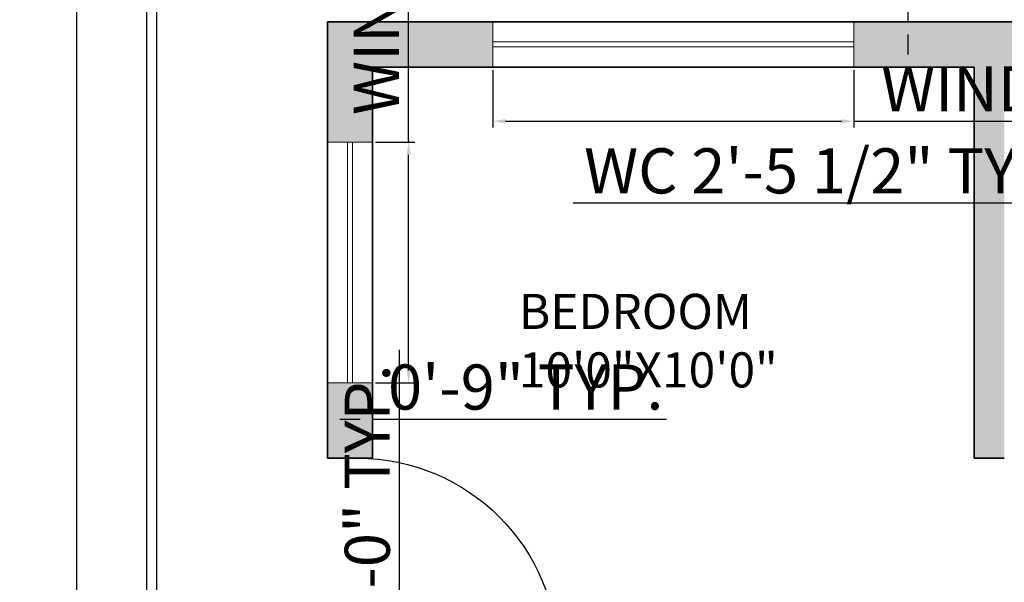
# Model space of a CAD drawing. Units: inches. Extents: x 2831 to 4250, y 1103 to 1797.
# Tile 3 of 15: x 3418 to 3614, y 1578 to 1690. Entities that reach past the tile are written whole.
import ezdxf

# ---------------------------------------------------------------- set-up
doc = ezdxf.new("R2010")
doc.units = ezdxf.units.IN
for name, color, linetype, lineweight in [('A-ANNO-DIMS', 2, 'Continuous', 18), ('A-AREA-IDEN', 7, 'Continuous', 18), ('A-DOOR', 4, 'Continuous', 25), ('A-WALL', 7, 'Continuous', 35), ('A-WALL-PATT', 252, 'Continuous', 13), ('C-PROP', 7, 'Continuous', 25), ('window', 130, 'Continuous', 18)]:
    doc.layers.add(name, color=color, linetype=linetype, lineweight=lineweight)
doc.styles.get("Standard").update_dxf_attribs({"font": 'arial.ttf'})
doc.dimstyles.new('ISO-25', dxfattribs={"dimtxt": 9, "dimasz": 2.5, "dimexe": 1.25, "dimexo": 0.625, "dimtad": 1, "dimdec": 1, "dimlunit": 3, "dimtxsty": 'Standard', "dimcen": 2.5, "dimadec": 0, "dimazin": 0, "dimtfac": 1, "dimtdec": 1, "dimtmove": 0, "dimatfit": 3, "dimfxl": 1, "dimarcsym": 0})

# ---------------------------------------------------------------- blocks, each defined once
blk = doc.blocks.new('*U2')
for p, q in [((0, 0), (0, -6)), ((40, 0), (40, -6))]:
    blk.add_line(p, q)
blk.add_lwpolyline([(0, 0), (0, 40), (1.75, 40), (1.75, 0)], close=True)
blk.add_arc((0, 0), 40, 0, 90)
blk = doc.blocks.new('*D6')
at = {"layer": 'A-ANNO-DIMS', "color": 0, "lineweight": -2, "transparency": 16777216}
for p, q in [((3442.6, 1722.51), (3427.96, 1722.51)), ((3429.21, 1720.01), (3429.21, 1245.01)), ((3442.6, 1242.51), (3427.96, 1242.51))]:
    blk.add_line(p, q, dxfattribs=at)
at = {"layer": 'A-ANNO-DIMS', "color": 0, "transparency": 16777216}
for points in [[(3428.79, 1720.01), (3429.62, 1720.01), (3429.21, 1722.51)], [(3428.79, 1245.01), (3429.62, 1245.01), (3429.21, 1242.51)]]:
    blk.add_solid(points, dxfattribs=at)
at = {"layer": 'Defpoints', "color": 0, "transparency": 16777216}
for p in [(3443.23, 1722.51), (3429.21, 1242.51), (3443.23, 1242.51)]:
    blk.add_point(p, dxfattribs=at)
at = {"layer": 'A-ANNO-DIMS', "color": 0, "transparency": 16777216, "insert": (3423.99, 1482.51), "char_height": 9, "attachment_point": 5, "rotation": 90}
blk.add_mtext("40'", dxfattribs=at)
blk = doc.blocks.new('WIN-48IN')
for p, q in [((9, 48), (0, 48)), ((4, 0), (4, 48)), ((5, 0), (5, 48)), ((9, 0), (0, 0))]:
    blk.add_line(p, q)
blk = doc.blocks.new('WIN-72IN')
for p, q in [((0, 0), (0, 9)), ((72, 0), (72, 9)), ((0, 5), (72, 5)), ((0, 4), (72, 4))]:
    blk.add_line(p, q)
blk = doc.blocks.new('*D73')
at = {"layer": 'A-ANNO-DIMS', "color": 0, "lineweight": -2, "transparency": 16777216}
for p, q in [((3495.43, 1665.51), (3495.43, 1783.15)), ((3488.85, 1665.51), (3496.68, 1665.51)), ((3495.43, 1620.01), (3495.43, 1663.01)), ((3488.85, 1617.51), (3496.68, 1617.51))]:
    blk.add_line(p, q, dxfattribs=at)
at = {"layer": 'A-ANNO-DIMS', "color": 0, "transparency": 16777216}
for points in [[(3495.01, 1663.01), (3495.84, 1663.01), (3495.43, 1665.51)], [(3495.01, 1620.01), (3495.84, 1620.01), (3495.43, 1617.51)]]:
    blk.add_solid(points, dxfattribs=at)
at = {"layer": 'Defpoints', "color": 0, "transparency": 16777216}
for p in [(3488.23, 1665.51), (3495.43, 1665.51), (3488.23, 1617.51)]:
    blk.add_point(p, dxfattribs=at)
at = {"layer": 'A-ANNO-DIMS', "color": 0, "transparency": 16777216, "insert": (3490.15, 1725.58), "char_height": 9, "attachment_point": 5, "rotation": 90}
blk.add_mtext('WINDOW 4\'-0" TYP.', dxfattribs=at)
blk = doc.blocks.new('*D74')
at = {"layer": 'A-ANNO-DIMS', "color": 0, "lineweight": -2, "transparency": 16777216}
for p, q in [((3479.23, 1616.89), (3479.23, 1609.06)), ((3488.23, 1616.89), (3488.23, 1609.06)), ((3481.73, 1610.31), (3485.73, 1610.31)), ((3488.23, 1610.31), (3546.84, 1610.31))]:
    blk.add_line(p, q, dxfattribs=at)
at = {"layer": 'A-ANNO-DIMS', "color": 0, "transparency": 16777216}
for points in [[(3481.73, 1610.73), (3481.73, 1609.9), (3479.23, 1610.31)], [(3485.73, 1610.73), (3485.73, 1609.9), (3488.23, 1610.31)]]:
    blk.add_solid(points, dxfattribs=at)
at = {"layer": 'Defpoints', "color": 0, "transparency": 16777216}
for p in [(3479.23, 1617.51), (3488.23, 1617.51), (3488.23, 1610.31)]:
    blk.add_point(p, dxfattribs=at)
at = {"layer": 'A-ANNO-DIMS', "color": 0, "transparency": 16777216, "insert": (3518.78, 1615.53), "char_height": 9, "attachment_point": 5}
blk.add_mtext('0\'-9" TYP.', dxfattribs=at)
blk = doc.blocks.new('*D75')
at = {"layer": 'A-ANNO-DIMS', "color": 0, "lineweight": -2, "transparency": 16777216}
for p, q in [((3493.63, 1506.51), (3493.63, 1624.15)), ((3488.85, 1506.51), (3494.88, 1506.51)), ((3493.63, 1473.01), (3493.63, 1504.01)), ((3488.85, 1470.51), (3494.88, 1470.51))]:
    blk.add_line(p, q, dxfattribs=at)
at = {"layer": 'A-ANNO-DIMS', "color": 0, "transparency": 16777216}
for points in [[(3493.21, 1504.01), (3494.04, 1504.01), (3493.63, 1506.51)], [(3493.21, 1473.01), (3494.04, 1473.01), (3493.63, 1470.51)]]:
    blk.add_solid(points, dxfattribs=at)
at = {"layer": 'Defpoints', "color": 0, "transparency": 16777216}
for p in [(3488.23, 1506.51), (3493.63, 1506.51), (3488.23, 1470.51)]:
    blk.add_point(p, dxfattribs=at)
at = {"layer": 'A-ANNO-DIMS', "color": 0, "transparency": 16777216, "insert": (3488.34, 1566.58), "char_height": 9, "attachment_point": 5, "rotation": 90}
blk.add_mtext('WINDOW 3\'-0" TYP.', dxfattribs=at)
blk = doc.blocks.new('*D77')
at = {"layer": 'A-ANNO-DIMS', "color": 0, "lineweight": -2, "transparency": 16777216}
for p, q in [((3512.23, 1679.89), (3512.23, 1668.46)), ((3584.23, 1679.89), (3584.23, 1668.46)), ((3514.73, 1669.71), (3581.73, 1669.71)), ((3584.23, 1669.71), (3701.86, 1669.71))]:
    blk.add_line(p, q, dxfattribs=at)
at = {"layer": 'A-ANNO-DIMS', "color": 0, "transparency": 16777216}
for points in [[(3514.73, 1670.13), (3514.73, 1669.3), (3512.23, 1669.71)], [(3581.73, 1670.13), (3581.73, 1669.3), (3584.23, 1669.71)]]:
    blk.add_solid(points, dxfattribs=at)
at = {"layer": 'Defpoints', "color": 0, "transparency": 16777216}
for p in [(3512.23, 1680.51), (3584.23, 1680.51), (3584.23, 1669.71)]:
    blk.add_point(p, dxfattribs=at)
at = {"layer": 'A-ANNO-DIMS', "color": 0, "transparency": 16777216, "insert": (3644.3, 1674.99), "char_height": 9, "attachment_point": 5}
blk.add_mtext('WINDOW 6\'-0" TYP.', dxfattribs=at)
blk = doc.blocks.new('*D78')
at = {"layer": 'A-ANNO-DIMS', "color": 0, "lineweight": -2, "transparency": 16777216}
for p, q in [((3595.03, 1689.51), (3595.03, 1748.12)), ((3584.85, 1689.51), (3596.28, 1689.51)), ((3595.03, 1683.01), (3595.03, 1687.01)), ((3584.85, 1680.51), (3596.28, 1680.51))]:
    blk.add_line(p, q, dxfattribs=at)
at = {"layer": 'A-ANNO-DIMS', "color": 0, "transparency": 16777216}
for points in [[(3594.61, 1687.01), (3595.44, 1687.01), (3595.03, 1689.51)], [(3594.61, 1683.01), (3595.44, 1683.01), (3595.03, 1680.51)]]:
    blk.add_solid(points, dxfattribs=at)
at = {"layer": 'Defpoints', "color": 0, "transparency": 16777216}
for p in [(3584.23, 1689.51), (3595.03, 1689.51), (3584.23, 1680.51)]:
    blk.add_point(p, dxfattribs=at)
at = {"layer": 'A-ANNO-DIMS', "color": 0, "transparency": 16777216, "insert": (3589.81, 1720.07), "char_height": 9, "attachment_point": 5, "rotation": 90}
blk.add_mtext('0\'-9" TYP.', dxfattribs=at)
blk = doc.blocks.new('*D89')
at = {"layer": 'A-ANNO-DIMS', "color": 0, "lineweight": -2, "transparency": 16777216}
for p, q in [((3632.62, 1657.17), (3632.62, 1652.11)), ((3662.23, 1657.17), (3662.23, 1652.11)), ((3632.62, 1653.36), (3528.23, 1653.36)), ((3659.73, 1653.36), (3635.12, 1653.36))]:
    blk.add_line(p, q, dxfattribs=at)
at = {"layer": 'A-ANNO-DIMS', "color": 0, "transparency": 16777216}
for points in [[(3635.12, 1653.77), (3635.12, 1652.94), (3632.62, 1653.36)], [(3659.73, 1653.77), (3659.73, 1652.94), (3662.23, 1653.36)]]:
    blk.add_solid(points, dxfattribs=at)
at = {"layer": 'Defpoints', "color": 0, "transparency": 16777216}
for p in [(3632.62, 1657.8), (3662.23, 1657.8), (3632.62, 1653.36)]:
    blk.add_point(p, dxfattribs=at)
at = {"layer": 'A-ANNO-DIMS', "color": 0, "transparency": 16777216, "insert": (3579.17, 1658.64), "char_height": 9, "attachment_point": 5}
blk.add_mtext('WC 2\'-5 1/2" TYP.', dxfattribs=at)

msp = doc.modelspace()

# ---------------------------------------------------------------- hatches: boundary and pattern name
at = {"layer": 'A-WALL-PATT'}
h = msp.add_hatch(color=256, dxfattribs=at)
h.dxf.hatch_style = 1
h.paths.add_polyline_path([(3479.23, 1418.51), (3488.23, 1418.51), (3488.23, 1426.81), (3488.23, 1460.51), (3588.23, 1460.51), (3588.23, 1466.51), (3488.23, 1466.51), (3488.23, 1470.51), (3479.23, 1470.51)])
h.paths.add_polyline_path([(3488.23, 1506.51), (3488.23, 1512.51), (3479.23, 1512.51), (3479.23, 1506.51)])
h.paths.add_polyline_path([(3488.23, 1370.51), (3479.23, 1370.51), (3479.23, 1319.51), (3521.23, 1319.51), (3521.23, 1328.51), (3488.23, 1328.51)])
h.paths.add_polyline_path([(3794.23, 1319.51), (3794.23, 1247.51), (3614.23, 1247.51), (3614.23, 1242.51), (3803.23, 1242.51), (3803.23, 1328.51), (3767.23, 1328.51), (3767.23, 1394.51), (3758.23, 1394.51), (3758.23, 1328.51), (3635.23, 1328.51), (3635.23, 1460.51), (3637.23, 1460.51), (3637.23, 1466.51), (3624.23, 1466.51), (3624.23, 1460.51), (3626.23, 1460.51), (3626.23, 1328.51), (3593.23, 1328.51), (3593.23, 1319.51)])
h.paths.add_polyline_path([(3758.23, 1460.51), (3758.23, 1442.51), (3767.23, 1442.51), (3767.23, 1460.51), (3783.23, 1460.51), (3783.23, 1492.51), (3774.23, 1492.51), (3774.23, 1466.51), (3761.32, 1466.51), (3726.23, 1466.51), (3726.23, 1468.51), (3720.23, 1468.51), (3720.23, 1466.51), (3673.23, 1466.51), (3673.23, 1460.51)])
h.paths.add_polyline_path([(3597.63, 1698.24), (3687.22, 1698.24), (3687.22, 1717.46), (3597.63, 1717.46)], flags=9)
h.paths.add_polyline_path([(3776.75, 1438.29), (3776.75, 1360.77), (3795.97, 1360.77), (3795.97, 1438.29)], flags=25)
h.paths.add_polyline_path([(3453.37, 1482.95), (3453.37, 1401.85), (3472.59, 1401.85), (3472.59, 1482.95)], flags=9)
h.paths.add_polyline_path([(3506.21, 1267.1), (3560.71, 1267.1), (3560.71, 1293.71), (3506.21, 1293.71)], flags=9)
h.paths.add_polyline_path([(3760.5, 1579.7), (3798.74, 1579.7), (3798.74, 1602.51), (3760.5, 1602.51)], flags=9)
h.paths.add_polyline_path([(3617, 1637.95), (3659.12, 1637.95), (3659.12, 1660.76), (3617, 1660.76)], flags=9)
h.paths.add_polyline_path([(3679.39, 1612.63), (3728.46, 1612.63), (3728.46, 1639.25), (3679.39, 1639.25)], flags=9)
h.paths.add_polyline_path([(3731.07, 1499.72), (3773.19, 1499.72), (3773.19, 1522.53), (3731.07, 1522.53)], flags=9)
h.paths.add_polyline_path([(3652.82, 1496.49), (3701.95, 1496.49), (3701.95, 1523.1), (3652.82, 1523.1)], flags=9)
h.paths.add_polyline_path([(3550.37, 1510.97), (3604.5, 1510.97), (3604.5, 1537.58), (3550.37, 1537.58)], flags=9)
h.paths.add_polyline_path([(3514.45, 1612.63), (3570.67, 1612.63), (3570.67, 1639.25), (3514.45, 1639.25)], flags=9)
h = msp.add_hatch(color=256, dxfattribs=at)
h.dxf.hatch_style = 1
h.paths.add_polyline_path([(3783.23, 1560.51), (3767.23, 1560.51), (3767.23, 1572.51), (3761.23, 1572.51), (3758.23, 1572.51), (3758.23, 1560.51), (3488.23, 1560.51), (3488.23, 1562.51), (3485.23, 1562.51), (3479.23, 1562.51), (3479.23, 1552.51), (3485.23, 1552.51), (3488.23, 1552.51), (3488.23, 1554.51), (3642.23, 1554.51), (3642.23, 1498.51), (3648.23, 1498.51), (3648.23, 1554.51), (3720.23, 1554.51), (3720.23, 1498.51), (3726.23, 1498.51), (3726.23, 1554.51), (3774.23, 1554.51), (3774.23, 1528.51), (3783.23, 1528.51)])
h.paths.add_polyline_path([(3767.23, 1689.51), (3728.23, 1689.51), (3728.23, 1680.51), (3758.23, 1680.51), (3758.23, 1602.51), (3767.23, 1602.51)])
h.paths.add_polyline_path([(3680.23, 1689.51), (3656.23, 1689.51), (3656.23, 1680.51), (3662.23, 1680.51), (3662.23, 1608.51), (3644.23, 1608.51), (3644.23, 1602.51), (3668.23, 1602.51), (3668.23, 1680.51), (3680.23, 1680.51)])
h.paths.add_polyline_path([(3620.23, 1689.51), (3584.23, 1689.51), (3584.23, 1680.51), (3608.23, 1680.51), (3608.23, 1602.51), (3614.23, 1602.51), (3614.23, 1608.51), (3614.23, 1638.51), (3614.23, 1680.51), (3620.23, 1680.51)])
h.paths.add_polyline_path([(3512.23, 1689.51), (3479.23, 1689.51), (3479.23, 1665.51), (3488.23, 1665.51), (3488.23, 1680.51), (3512.23, 1680.51)])
h.paths.add_polyline_path([(3488.23, 1617.51), (3479.23, 1617.51), (3479.23, 1602.51), (3485.23, 1602.51), (3488.23, 1602.51)])

# ---------------------------------------------------------------- linework, layer by layer
at = {"layer": 'A-WALL'}
for p, q in [((3479.23, 1689.51), (3803.23, 1689.51)), ((3479.23, 1602.51), (3479.23, 1689.51)), ((3488.23, 1680.51), (3608.23, 1680.51)), ((3488.23, 1602.51), (3488.23, 1680.51)), ((3608.23, 1602.51), (3608.23, 1680.51)), ((3479.23, 1602.51), (3488.23, 1602.51)), ((3608.23, 1602.51), (3614.23, 1602.51))]:
    msp.add_line(p, q, dxfattribs=at)
at = {"layer": 'C-PROP'}
msp.add_lwpolyline([(3443.23, 1722.51), (3803.23, 1722.51), (3803.23, 1242.51), (3443.23, 1242.51)], close=True, dxfattribs=at)
msp.add_lwpolyline([(3445.23, 1244.51), (3445.23, 1720.51), (3801.23, 1720.51)], dxfattribs=at)

# ---------------------------------------------------------------- block references
at = {"layer": 'A-DOOR', "xscale": -1, "rotation": 270}
msp.add_blockref('*U2', (3485.23, 1562.51), dxfattribs=at)
at = {"layer": 'window'}
for name, p in [('WIN-72IN', (3512.23, 1680.51)), ('WIN-48IN', (3479.23, 1617.51))]:
    msp.add_blockref(name, p, dxfattribs=at)

# ---------------------------------------------------------------- texts
at = {"layer": 'A-AREA-IDEN', "insert": (3517.41, 1635.28), "char_height": 7, "attachment_point": 1}
msp.add_mtext_dynamic_manual_height_columns('{\\fTimes New Roman|b0|i0|c0|p18;BEDROOM\\P10\'0"X10\'0"}', width=81.5075, gutter_width=12.5, heights=[0], dxfattribs=at)

# ---------------------------------------------------------------- dimensions: what is measured, and where the dimension line sits
at = {"layer": 'A-ANNO-DIMS'}
for base, p1, p2, angle, text, picture, middle in [((3495.43, 1665.51), (3488.23, 1617.51), (3488.23, 1665.51), 90, 'WINDOW <> TYP.', '*D73', (3490.15, 1725.58)), ((3595.03, 1689.51), (3584.23, 1680.51), (3584.23, 1689.51), 90, '<> TYP.', '*D78', (3589.81, 1720.07)), ((3632.62, 1653.36), (3662.23, 1657.8), (3632.62, 1657.8), 180, 'WC <> TYP.', '*D89', (3579.17, 1658.64)), ((3493.63, 1506.51), (3488.23, 1470.51), (3488.23, 1506.51), 90, 'WINDOW <> TYP.', '*D75', (3488.34, 1566.58))]:
    dim = msp.add_linear_dim(base=base, p1=p1, p2=p2, angle=angle, text=text, dimstyle='ISO-25', override={"dimdec": 1, "dimlfac": 1, "dimrnd": 0, "dimzin": 1, "dimdsep": 46, "dimlunit": 4, "dimfrac": 2}, dxfattribs=at)
    dim.commit()
    dim.dimension.update_dxf_attribs({"geometry": picture, "text_midpoint": middle})
dim = msp.add_linear_dim(base=(3429.21, 1242.51), p1=(3443.23, 1722.51), p2=(3443.23, 1242.51), angle=90, dimstyle='ISO-25', override={"dimclrd": 0, "dimclre": 0, "dimclrt": 0}, dxfattribs=at)
dim.commit()
dim.dimension.update_dxf_attribs({"geometry": '*D6', "text_midpoint": (3423.99, 1482.51)})
for base, p1, p2, text, picture, middle in [((3584.23, 1669.71), (3512.23, 1680.51), (3584.23, 1680.51), 'WINDOW <> TYP.', '*D77', (3644.3, 1674.99)), ((3488.23, 1610.31), (3479.23, 1617.51), (3488.23, 1617.51), '<> TYP.', '*D74', (3518.78, 1615.53))]:
    dim = msp.add_linear_dim(base=base, p1=p1, p2=p2, text=text, dimstyle='ISO-25', override={"dimdec": 1, "dimlfac": 1, "dimrnd": 0, "dimzin": 1, "dimdsep": 46, "dimlunit": 4, "dimfrac": 2}, dxfattribs=at)
    dim.commit()
    dim.dimension.update_dxf_attribs({"geometry": picture, "text_midpoint": middle})

doc.saveas('drawing.dxf')
